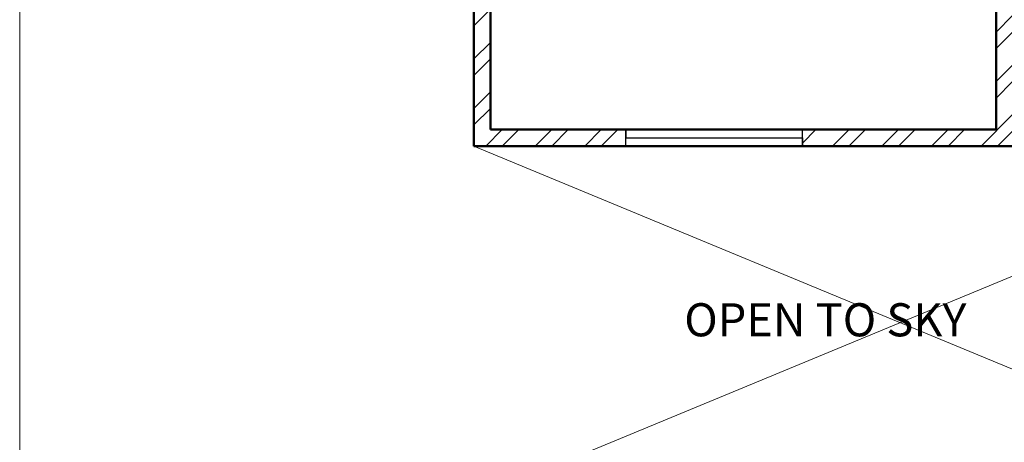
# Model space of a CAD drawing. Units: inches. Extents: x 1901 to 2863, y 888 to 2433.
# Tile 49 of 91: x 1901 to 2169, y 1732 to 1847. Entities that reach past the tile are written whole.
import ezdxf

# ---------------------------------------------------------------- set-up
doc = ezdxf.new("R2010")
doc.units = ezdxf.units.IN
for name, color, linetype, lineweight in [('A-ANNO-SYMB', 8, 'Continuous', 13), ('A-AREA-IDEN', 7, 'Continuous', 18), ('A-FLOR-FIXT', 9, 'Continuous', 18), ('A-GLAZ', 3, 'Continuous', 25), ('A-WALL', 7, 'Continuous', 50), ('A-WALL-PATT', 8, 'Continuous', 13)]:
    doc.layers.add(name, color=color, linetype=linetype, lineweight=lineweight)
doc.styles.get("Standard").update_dxf_attribs({"font": 'arial.ttf'})

# ---------------------------------------------------------------- blocks, each defined once
blk = doc.blocks.new('WIN-48')
for p, q in [((0, 2.25), (0, 4.5)), ((0, 4.5), (0, 0)), ((48, 4.5), (48, 0)), ((48, 2.25), (0, 2.25)), ((48, 0), (48, 2.25))]:
    blk.add_line(p, q)

msp = doc.modelspace()

# ---------------------------------------------------------------- hatches: boundary and pattern name
at = {"layer": 'A-WALL-PATT'}
h = msp.add_hatch(dxfattribs=at)
h.set_pattern_fill('ANSI32', color=256)
h.paths.add_polyline_path([(2192.5, 2274.13), (2141.26, 2274.13), (2141.26, 2269.63), (2192.5, 2269.63)])
h.paths.add_polyline_path([(2259.93, 2274.13), (2216.5, 2274.13), (2216.5, 2269.63), (2255.43, 2269.63), (2255.43, 2214.63), (2250.81, 2214.63), (2250.81, 2210.13), (2259.93, 2210.13), (2259.93, 2215.13), (2271.76, 2215.13), (2271.76, 2217.38), (2271.76, 2219.63), (2259.93, 2219.63)])
h.paths.add_polyline_path([(2171.43, 2269.63), (2166.93, 2269.63), (2166.93, 2219.63), (2121.24, 2219.63), (2121.24, 2215.13), (2166.93, 2215.13), (2166.93, 2083.13), (2161.81, 2083.13), (2161.81, 2078.63), (2171.43, 2078.63), (2177, 2078.63), (2177, 2080.88), (2177, 2083.13), (2171.43, 2083.13), (2171.43, 2210.13), (2230.91, 2210.13), (2230.91, 2212.38), (2230.91, 2214.63), (2171.43, 2214.63)])
h.paths.add_polyline_path([(2117.26, 2274.13), (2089.43, 2274.13), (2089.43, 2219.63), (2081.14, 2219.63), (2081.14, 2215.13), (2089.43, 2215.13), (2098, 2215.13), (2098, 2217.38), (2098, 2219.63), (2093.93, 2219.63), (2093.93, 2269.63), (2117.26, 2269.63), (2117.26, 2271.88)])
h.paths.add_polyline_path([(2343.43, 2219.63), (2329.29, 2219.63), (2329.29, 2215.13), (2338.93, 2215.13), (2338.93, 2184.74), (2343.43, 2184.74)])
h.paths.add_polyline_path([(2338.93, 2083.13), (2329.29, 2083.13), (2208.97, 2083.13), (2208.97, 2078.63), (2338.93, 2078.63)])
h.paths.add_polyline_path([(2343.43, 2136.74), (2338.93, 2136.74), (2338.93, 1872.63), (2343.43, 1872.63)])
h.paths.add_polyline_path([(2343.43, 1863.63), (2397.68, 1863.63), (2397.68, 1821.63), (2384.14, 1821.63), (2384.14, 1812.63), (2418.33, 1812.63), (2418.33, 1817.13), (2418.33, 1821.63), (2406.68, 1821.63), (2406.68, 1863.63), (2459.5, 1863.63), (2459.5, 1821.63), (2447.14, 1821.63), (2447.14, 1812.63), (2459.5, 1812.63), (2468.5, 1812.63), (2468.5, 1872.63), (2394.43, 1872.63), (2334.43, 1872.63), (2334.43, 1812.63), (2343.43, 1812.63), (2353.25, 1812.63), (2353.25, 1821.63), (2343.43, 1821.63)])
h.paths.add_polyline_path([(2510.01, 1872.63), (2468.5, 1872.63), (2468.5, 1868.13), (2510.01, 1868.13)])
h.paths.add_polyline_path([(2514.01, 1817.13), (2468.5, 1817.13), (2468.5, 1812.63), (2482.11, 1812.63), (2482.11, 1800.61), (2486.61, 1800.61), (2486.61, 1812.63), (2514.01, 1812.63)])
h.paths.add_polyline_path([(2299.25, 1814.88), (2299.25, 1817.13), (2295.93, 1817.13), (2295.93, 1854.17), (2293.68, 1854.17), (2291.43, 1854.17), (2291.43, 1817.13), (2266.11, 1817.13), (2266.11, 1812.63), (2299.25, 1812.63)])
h.paths.add_polyline_path([(2218.11, 1817.13), (2206.46, 1817.13), (2171.43, 1817.13), (2171.43, 1949.13), (2190.1, 1949.13), (2190.1, 1953.63), (2163.47, 1953.63), (2163.47, 1949.13), (2166.93, 1949.13), (2166.93, 1817.13), (2114.3, 1817.13), (2114.3, 1812.63), (2218.11, 1812.63)])
h.paths.add_polyline_path([(2029.43, 1970.92), (2024.93, 1970.92), (2024.93, 1912.72), (2029.43, 1912.72)])
h.paths.add_polyline_path([(2132.3, 1953.63), (2113.93, 1953.63), (2113.93, 1975.89), (2111.68, 1975.89), (2109.43, 1975.89), (2109.43, 1953.63), (2029.43, 1953.63), (2029.43, 1949.13), (2132.3, 1949.13)])
h.paths.add_polyline_path([(2029.43, 1853.61), (2029.31, 1853.61), (2029.31, 1853.61), (2029.43, 1853.61), (2029.43, 1864.72), (2024.93, 1864.72), (2024.93, 1812.63), (2066.3, 1812.63), (2066.3, 1814.88), (2066.3, 1817.13), (2029.43, 1817.13)])
h.paths.add_polyline_path([(2122.93, 2010.09), (2120.68, 2010.09), (2118.43, 2010.09), (2118.43, 2006.13), (2029.43, 2006.13), (2029.43, 2001.63), (2109.43, 2001.63), (2109.43, 1998.04), (2113.93, 1998.04), (2113.93, 2001.63), (2122.93, 2001.63)])
h.paths.add_polyline_path([(2029.43, 2031.38), (2024.93, 2031.38), (2024.93, 1994.92), (2027.18, 1994.92), (2029.43, 1994.92)])
h.paths.add_polyline_path([(2029.43, 2136.74), (2024.93, 2136.74), (2024.93, 2067.38), (2027.18, 2067.38), (2029.43, 2067.38)])
h.paths.add_polyline_path([(2125.62, 2083.13), (2029.43, 2083.13), (2029.43, 2078.63), (2118.43, 2078.63), (2118.43, 2030.71), (2122.93, 2030.71), (2122.93, 2078.63), (2125.62, 2078.63)])
h.paths.add_polyline_path([(2029.43, 2215.13), (2040.47, 2215.13), (2040.47, 2217.38), (2040.47, 2219.63), (2024.93, 2219.63), (2024.93, 2184.74), (2029.43, 2184.74), (2029.43, 2187.78)])
h.paths.add_polyline_path([(2686.43, 2274.13), (2659.28, 2274.13), (2659.28, 2269.63), (2681.93, 2269.63), (2681.93, 2219.63), (2676.82, 2219.63), (2676.82, 2215.13), (2681.93, 2215.13), (2697.01, 2215.13), (2697.01, 2217.38), (2697.01, 2219.63), (2686.43, 2219.63)])
h.paths.add_polyline_path([(2609.93, 2269.63), (2635.28, 2269.63), (2635.28, 2274.13), (2571.43, 2274.13), (2571.43, 2269.63), (2605.43, 2269.63), (2605.43, 2214.63), (2549.1, 2214.63), (2549.1, 2210.13), (2605.43, 2210.13), (2605.43, 2083.13), (2601.01, 2083.13), (2601.01, 2080.88), (2601.01, 2078.63), (2609.93, 2078.63), (2616.16, 2078.63), (2616.16, 2080.88), (2616.16, 2083.13), (2609.93, 2083.13), (2609.93, 2215.13), (2651.46, 2215.13), (2651.46, 2217.38), (2651.46, 2219.63), (2609.93, 2219.63)])
h.paths.add_polyline_path([(2521.43, 2269.63), (2547.43, 2269.63), (2547.43, 2271.88), (2547.43, 2274.13), (2516.93, 2274.13), (2516.93, 2219.63), (2506.41, 2219.63), (2506.41, 2215.13), (2516.93, 2215.13), (2516.93, 2210.13), (2525.4, 2210.13), (2525.4, 2212.38), (2525.4, 2214.63), (2521.43, 2214.63)])
h.paths.add_polyline_path([(2456.01, 2219.63), (2439.43, 2219.63), (2439.43, 2187.89), (2443.93, 2187.89), (2443.93, 2215.13), (2456.01, 2215.13)])
h.paths.add_polyline_path([(2752.93, 2219.63), (2739.48, 2219.63), (2739.48, 2215.13), (2748.43, 2215.13), (2748.43, 2187.89), (2752.93, 2187.89)])
h.paths.add_polyline_path([(2752.93, 2139.89), (2748.43, 2139.89), (2748.43, 2083.13), (2648.42, 2083.13), (2648.42, 2078.63), (2654.93, 2078.63), (2654.93, 2039.44), (2659.43, 2039.44), (2659.43, 2078.63), (2748.43, 2078.63), (2748.43, 2063.43), (2752.93, 2063.43)])
h.paths.add_polyline_path([(2752.93, 2010.63), (2659.43, 2010.63), (2659.43, 2015.65), (2654.93, 2015.65), (2654.93, 2010.63), (2605.43, 2010.63), (2605.43, 1920.97), (2609.93, 1920.97), (2609.93, 2006.13), (2748.43, 2006.13), (2748.43, 1982.47), (2752.93, 1982.47)])
h.paths.add_polyline_path([(2752.93, 2027.43), (2748.43, 2027.43), (2748.43, 2010.63), (2752.93, 2010.63)])
h.paths.add_polyline_path([(2748.43, 1886.13), (2609.93, 1886.13), (2609.93, 1889.72), (2605.43, 1889.72), (2605.43, 1861.26), (2609.93, 1861.26), (2609.93, 1881.63), (2748.43, 1881.63)])
h.paths.add_polyline_path([(2456.86, 2228.83), (2498.4, 2228.83), (2498.4, 2247.49), (2456.86, 2247.49)], flags=9)
h.paths.add_polyline_path([(2038.6, 2237.42), (2080.17, 2237.42), (2080.17, 2256.08), (2038.6, 2256.08)], flags=9)
h.paths.add_polyline_path([(2292.01, 1062.39), (2539.93, 1062.39), (2539.93, 1099.49), (2292.01, 1099.49)], flags=9)
h.paths.add_polyline_path([(2424.91, 1832.25), (2448.51, 1832.25), (2448.51, 1846.68), (2424.91, 1846.68)], flags=25)
h.paths.add_polyline_path([(2359.08, 1832.25), (2382.68, 1832.25), (2382.68, 1846.68), (2359.08, 1846.68)], flags=25)
h.paths.add_polyline_path([(2352.9, 1684.8), (2367.54, 1684.8), (2367.54, 1697.17), (2352.9, 1697.17)], flags=9)
h.paths.add_polyline_path([(2079.29, 1755.83), (2169.02, 1755.83), (2169.02, 1774.37), (2079.29, 1774.37)], flags=9)
h.paths.add_polyline_path([(2404.09, 1373.86), (2404.09, 1463.59), (2385.54, 1463.59), (2385.54, 1373.86)], flags=9)
h.paths.add_polyline_path([(2268.09, 2236.37), (2309.64, 2236.37), (2309.64, 2255.03), (2268.09, 2255.03)], flags=9)
h.paths.add_polyline_path([(2575.96, 1700.95), (2665.7, 1700.95), (2665.7, 1719.5), (2575.96, 1719.5)], flags=9)
h.paths.add_polyline_path([(2302.96, 1878.47), (2329.52, 1878.47), (2329.52, 1888.78), (2302.96, 1888.78)], flags=9)
h.paths.add_polyline_path([(2097.42, 2240.58), (2126.57, 2240.58), (2126.57, 2259.23), (2097.42, 2259.23)], flags=9)
h.paths.add_polyline_path([(2208.72, 2246.12), (2237.88, 2246.12), (2237.88, 2264.78), (2208.72, 2264.78)], flags=9)
h.paths.add_polyline_path([(2038.15, 1925.96), (2076.99, 1925.96), (2076.99, 1944.62), (2038.15, 1944.62)], flags=9)
h.paths.add_polyline_path([(2239.14, 1926.67), (2288.46, 1926.67), (2288.46, 1945.33), (2239.14, 1945.33)], flags=9)
h.paths.add_polyline_path([(2175.43, 2007.33), (2212.36, 2007.33), (2212.36, 2025.99), (2175.43, 2025.99)], flags=9)
h.paths.add_polyline_path([(2225.03, 2091.79), (2263.87, 2091.79), (2263.87, 2110.45), (2225.03, 2110.45)], flags=9)
h.paths.add_polyline_path([(2035.4, 2098.48), (2074.24, 2098.48), (2074.24, 2117.14), (2035.4, 2117.14)], flags=9)
h.paths.add_polyline_path([(2050.1, 2029.21), (2083.26, 2029.21), (2083.26, 2047.87), (2050.1, 2047.87)], flags=9)
h.paths.add_polyline_path([(2069.68, 1956.72), (2098.83, 1956.72), (2098.83, 1975.38), (2069.68, 1975.38)], flags=25)
h.paths.add_polyline_path([(2328.62, 1753.34), (2361.66, 1753.34), (2361.66, 1771.99), (2328.62, 1771.99)], flags=9)
h.paths.add_polyline_path([(2395.16, 2060.89), (2395.16, 2140.65), (2378.68, 2140.65), (2378.68, 2060.89)], flags=9)
h.paths.add_polyline_path([(2463.73, 2059.02), (2492.89, 2059.02), (2492.89, 2077.68), (2463.73, 2077.68)], flags=9)
h.paths.add_polyline_path([(2458.03, 2181.54), (2496.87, 2181.54), (2496.87, 2200.19), (2458.03, 2200.19)], flags=9)
h.paths.add_polyline_path([(2527.58, 2243.07), (2556.73, 2243.07), (2556.73, 2261.73), (2527.58, 2261.73)], flags=9)
h.paths.add_polyline_path([(2694.46, 2232.77), (2736.03, 2232.77), (2736.03, 2251.42), (2694.46, 2251.42)], flags=9)
h.paths.add_polyline_path([(2637.82, 2249.22), (2666.98, 2249.22), (2666.98, 2267.88), (2637.82, 2267.88)], flags=9)
h.paths.add_polyline_path([(2623.69, 2183.54), (2662.53, 2183.54), (2662.53, 2202.2), (2623.69, 2202.2)], flags=9)
h.paths.add_polyline_path([(2691.97, 2021.5), (2725.12, 2021.5), (2725.12, 2040.16), (2691.97, 2040.16)], flags=9)
h.paths.add_polyline_path([(2621.04, 1975.91), (2662.34, 1975.91), (2662.34, 1994.57), (2621.04, 1994.57)], flags=25)
h.paths.add_polyline_path([(2479.03, 1927.62), (2519.84, 1927.62), (2519.84, 1946.28), (2479.03, 1946.28)], flags=9)
h.paths.add_polyline_path([(2670.94, 1849.08), (2716.01, 1849.08), (2716.01, 1867.73), (2670.94, 1867.73)], flags=9)
h.paths.add_polyline_path([(2523.61, 1782.96), (2550.17, 1782.96), (2550.17, 1793.26), (2523.61, 1793.26)], flags=9)
h.paths.add_polyline_path([(2450.84, 1207.33), (2492.39, 1207.33), (2492.39, 1225.99), (2450.84, 1225.99)], flags=9)
h.paths.add_polyline_path([(2527.75, 1203.84), (2556.91, 1203.84), (2556.91, 1222.5), (2527.75, 1222.5)], flags=9)
h.paths.add_polyline_path([(2639.11, 1207.2), (2668.27, 1207.2), (2668.27, 1225.86), (2639.11, 1225.86)], flags=9)
h.paths.add_polyline_path([(2692.59, 1218.97), (2734.17, 1218.97), (2734.17, 1237.62), (2692.59, 1237.62)], flags=9)
h.paths.add_polyline_path([(2669.27, 1366.33), (2708.11, 1366.33), (2708.11, 1384.99), (2669.27, 1384.99)], flags=9)
h.paths.add_polyline_path([(2463.31, 1358.03), (2502.15, 1358.03), (2502.15, 1376.69), (2463.31, 1376.69)], flags=9)
h.paths.add_polyline_path([(2494.72, 1449.96), (2531.65, 1449.96), (2531.65, 1468.62), (2494.72, 1468.62)], flags=9)
h.paths.add_polyline_path([(2675.57, 1422.16), (2708.72, 1422.16), (2708.72, 1440.81), (2675.57, 1440.81)], flags=9)
h.paths.add_polyline_path([(2685.63, 1493.89), (2714.79, 1493.89), (2714.79, 1512.55), (2685.63, 1512.55)], flags=9)
h.paths.add_polyline_path([(2686.8, 1529.91), (2725.65, 1529.91), (2725.65, 1548.57), (2686.8, 1548.57)], flags=9)
h.paths.add_polyline_path([(2503.65, 1537.99), (2552.97, 1537.99), (2552.97, 1556.65), (2503.65, 1556.65)], flags=9)
h.paths.add_polyline_path([(2291.71, 1643.5), (2318.28, 1643.5), (2318.28, 1653.81), (2291.71, 1653.81)], flags=9)
h.paths.add_polyline_path([(2450.63, 1610.52), (2477.19, 1610.52), (2477.19, 1620.82), (2450.63, 1620.82)], flags=9)
h.paths.add_polyline_path([(2359.99, 1551.81), (2422.25, 1551.81), (2422.25, 1562.12), (2359.99, 1562.12)], flags=9)
h.paths.add_polyline_path([(2280.11, 1249.01), (2321.65, 1249.01), (2321.65, 1267.66), (2280.11, 1267.66)], flags=9)
h.paths.add_polyline_path([(2164.06, 1274.23), (2193.22, 1274.23), (2193.22, 1292.89), (2164.06, 1292.89)], flags=9)
h.paths.add_polyline_path([(2118.21, 1277.69), (2151.25, 1277.69), (2151.25, 1296.35), (2118.21, 1296.35)], flags=9)
h.paths.add_polyline_path([(2031.95, 1268.53), (2073.52, 1268.53), (2073.52, 1287.19), (2031.95, 1287.19)], flags=9)
h.paths.add_polyline_path([(2050.2, 1409.08), (2089.04, 1409.08), (2089.04, 1427.74), (2050.2, 1427.74)], flags=9)
h.paths.add_polyline_path([(2243.74, 1421.03), (2282.58, 1421.03), (2282.58, 1439.69), (2243.74, 1439.69)], flags=9)
h.paths.add_polyline_path([(2190.75, 1509.77), (2231.56, 1509.77), (2231.56, 1528.43), (2190.75, 1528.43)], flags=9)
h.paths.add_polyline_path([(2058.39, 1475.42), (2091.55, 1475.42), (2091.55, 1494.07), (2058.39, 1494.07)], flags=9)
h.paths.add_polyline_path([(2062.45, 1553.09), (2091.6, 1553.09), (2091.6, 1571.75), (2062.45, 1571.75)], flags=9)
h.paths.add_polyline_path([(2219.52, 1590.37), (2266.15, 1590.37), (2266.15, 1609.02), (2219.52, 1609.02)], flags=9)
h.paths.add_polyline_path([(2041.07, 1584.19), (2079.91, 1584.19), (2079.91, 1602.85), (2041.07, 1602.85)], flags=9)
h = msp.add_hatch(dxfattribs=at)
h.set_pattern_fill('ANSI32', color=256)
h.paths.add_polyline_path([(2443.93, 2139.89), (2439.43, 2139.89), (2439.43, 2069.35), (2441.68, 2069.35), (2443.93, 2069.35), (2443.93, 2078.63), (2521.93, 2078.63), (2521.93, 2075.07), (2524.18, 2075.07), (2526.43, 2075.07), (2526.43, 2078.63), (2571.75, 2078.63), (2571.75, 2080.88), (2571.75, 2083.13), (2443.93, 2083.13)])
h.paths.add_polyline_path([(2526.43, 2054.63), (2524.18, 2054.63), (2521.93, 2054.63), (2521.93, 2030.63), (2443.93, 2030.63), (2443.93, 2045.35), (2439.43, 2045.35), (2439.43, 1983.87), (2443.93, 1983.87), (2443.93, 2026.13), (2521.93, 2026.13), (2526.43, 2026.13)])
h.paths.add_polyline_path([(2443.93, 1923.87), (2439.43, 1923.87), (2439.43, 1872.63), (2443.93, 1872.63)])
h.paths.add_polyline_path([(2636.23, 1766.13), (2609.93, 1766.13), (2609.93, 1779.79), (2605.43, 1779.79), (2605.43, 1766.13), (2486.61, 1766.13), (2486.61, 1770.67), (2482.11, 1770.67), (2482.11, 1766.13), (2482.11, 1761.63), (2636.23, 1761.63), (2636.23, 1763.88)])
h.paths.add_polyline_path([(2519.54, 1663.38), (2519.54, 1665.63), (2494.93, 1665.63), (2481.83, 1665.63), (2481.83, 1663.38), (2481.83, 1661.13), (2490.43, 1661.13), (2490.43, 1640.16), (2494.93, 1640.16), (2494.93, 1661.13), (2519.54, 1661.13)])
h.paths.add_polyline_path([(2443.93, 1712.13), (2443.93, 1716.63), (2414.46, 1716.63), (2414.46, 1712.13), (2439.43, 1712.13), (2439.43, 1545.51), (2443.93, 1545.51), (2443.93, 1661.13), (2448.47, 1661.13), (2448.47, 1665.63), (2443.93, 1665.63)])
h.paths.add_polyline_path([(2343.43, 1712.13), (2365.52, 1712.13), (2365.52, 1714.38), (2365.52, 1716.63), (2333.87, 1716.63), (2333.87, 1714.38), (2333.87, 1712.13), (2338.93, 1712.13), (2338.93, 1575.63), (2338.93, 1545.51), (2343.43, 1545.51), (2343.43, 1547.51), (2343.43, 1580.13)])
h.paths.add_polyline_path([(2752.93, 1665.63), (2579.54, 1665.63), (2579.54, 1661.13), (2615.93, 1661.13), (2615.93, 1529.13), (2598.93, 1529.13), (2598.93, 1524.63), (2623.13, 1524.63), (2623.13, 1526.88), (2623.13, 1529.13), (2620.43, 1529.13), (2620.43, 1661.13), (2748.43, 1661.13), (2748.43, 1633.5), (2752.93, 1633.5)])
h.paths.add_polyline_path([(2752.93, 1419.93), (2748.43, 1419.93), (2748.43, 1400.13), (2659.43, 1400.13), (2659.43, 1444.33), (2657.18, 1444.33), (2654.93, 1444.33), (2654.93, 1400.13), (2643.65, 1400.13), (2643.65, 1395.63), (2748.43, 1395.63), (2748.43, 1364.04), (2752.93, 1364.04)])
h.paths.add_polyline_path([(2752.93, 1492.88), (2748.43, 1492.88), (2748.43, 1476.63), (2667.43, 1476.63), (2667.43, 1479.71), (2665.18, 1479.71), (2662.93, 1479.71), (2662.93, 1476.63), (2654.93, 1476.63), (2654.93, 1469.54), (2659.43, 1469.54), (2659.43, 1472.13), (2748.43, 1472.13), (2748.43, 1455.93), (2752.93, 1455.93)])
h.paths.add_polyline_path([(2752.93, 1304.04), (2748.43, 1304.04), (2748.43, 1263.63), (2738.66, 1263.63), (2738.66, 1259.13), (2752.93, 1259.13)])
h.paths.add_polyline_path([(2685.93, 1259.13), (2695.49, 1259.13), (2695.49, 1261.38), (2695.49, 1263.63), (2677.84, 1263.63), (2677.84, 1261.38), (2677.84, 1259.13), (2681.43, 1259.13), (2681.43, 1203.63), (2653.28, 1203.63), (2653.28, 1199.13), (2685.93, 1199.13), (2685.93, 1203.63)])
h.paths.add_polyline_path([(2609.43, 1395.63), (2611.85, 1395.63), (2611.85, 1400.13), (2598.89, 1400.13), (2598.89, 1397.88), (2598.89, 1395.63), (2604.93, 1395.63), (2604.93, 1268.13), (2554.73, 1268.13), (2554.73, 1265.88), (2554.73, 1263.63), (2604.93, 1263.63), (2604.93, 1203.63), (2571.31, 1203.63), (2571.31, 1199.13), (2604.93, 1199.13), (2629.28, 1199.13), (2629.28, 1201.38), (2629.28, 1203.63), (2609.43, 1203.63), (2609.43, 1258.63), (2609.43, 1259.13), (2654.8, 1259.13), (2654.8, 1263.63), (2609.43, 1263.63)])
h.paths.add_polyline_path([(2443.93, 1304.04), (2439.43, 1304.04), (2439.43, 1259.13), (2443.93, 1259.13), (2456.16, 1259.13), (2456.16, 1261.38), (2456.16, 1263.63), (2443.93, 1263.63)])
h.paths.add_polyline_path([(2525.43, 1263.63), (2531.78, 1263.63), (2531.78, 1268.13), (2520.93, 1268.13), (2520.93, 1263.63), (2511.41, 1263.63), (2511.41, 1259.13), (2520.93, 1259.13), (2520.93, 1199.13), (2547.31, 1199.13), (2547.31, 1201.38), (2547.31, 1203.63), (2525.43, 1203.63)])
h.paths.add_polyline_path([(2443.93, 1434.84), (2439.43, 1434.84), (2439.43, 1364.04), (2441.68, 1364.04), (2443.93, 1364.04)])
h.paths.add_polyline_path([(2567.13, 1400.13), (2443.93, 1400.13), (2443.93, 1395.63), (2567.13, 1395.63)])
h.paths.add_polyline_path([(2443.93, 1545.51), (2439.43, 1545.51), (2439.43, 1494.84), (2443.93, 1494.84)])
h.paths.add_polyline_path([(2494.93, 1553.35), (2492.68, 1553.35), (2490.43, 1553.35), (2490.43, 1524.63), (2494.93, 1524.63), (2525.94, 1524.63), (2525.94, 1526.88), (2525.94, 1529.13), (2494.93, 1529.13)])
h.paths.add_polyline_path([(2752.93, 1573.5), (2748.43, 1573.5), (2748.43, 1529.13), (2657.76, 1529.13), (2657.76, 1524.63), (2662.93, 1524.63), (2662.93, 1498.63), (2667.43, 1498.63), (2667.43, 1524.63), (2748.43, 1524.63), (2748.43, 1516.88), (2752.93, 1516.88)])
h.paths.add_polyline_path([(2038.6, 2237.42), (2080.17, 2237.42), (2080.17, 2256.08), (2038.6, 2256.08)], flags=9)
h.paths.add_polyline_path([(2292.01, 1062.39), (2539.93, 1062.39), (2539.93, 1099.49), (2292.01, 1099.49)], flags=9)
h.paths.add_polyline_path([(2424.91, 1832.25), (2448.51, 1832.25), (2448.51, 1846.68), (2424.91, 1846.68)], flags=9)
h.paths.add_polyline_path([(2359.08, 1832.25), (2382.68, 1832.25), (2382.68, 1846.68), (2359.08, 1846.68)], flags=9)
h.paths.add_polyline_path([(2352.9, 1684.8), (2367.54, 1684.8), (2367.54, 1697.17), (2352.9, 1697.17)], flags=9)
h.paths.add_polyline_path([(2079.29, 1755.83), (2169.02, 1755.83), (2169.02, 1774.37), (2079.29, 1774.37)], flags=9)
h.paths.add_polyline_path([(2404.09, 1373.86), (2404.09, 1463.59), (2385.54, 1463.59), (2385.54, 1373.86)], flags=9)
h.paths.add_polyline_path([(2268.09, 2236.37), (2309.64, 2236.37), (2309.64, 2255.03), (2268.09, 2255.03)], flags=9)
h.paths.add_polyline_path([(2575.96, 1700.95), (2665.7, 1700.95), (2665.7, 1719.5), (2575.96, 1719.5)], flags=9)
h.paths.add_polyline_path([(2302.96, 1878.47), (2329.52, 1878.47), (2329.52, 1888.78), (2302.96, 1888.78)], flags=9)
h.paths.add_polyline_path([(2097.42, 2240.58), (2126.57, 2240.58), (2126.57, 2259.23), (2097.42, 2259.23)], flags=9)
h.paths.add_polyline_path([(2208.72, 2246.12), (2237.88, 2246.12), (2237.88, 2264.78), (2208.72, 2264.78)], flags=9)
h.paths.add_polyline_path([(2038.15, 1925.96), (2076.99, 1925.96), (2076.99, 1944.62), (2038.15, 1944.62)], flags=9)
h.paths.add_polyline_path([(2239.14, 1926.67), (2288.46, 1926.67), (2288.46, 1945.33), (2239.14, 1945.33)], flags=9)
h.paths.add_polyline_path([(2175.43, 2007.33), (2212.36, 2007.33), (2212.36, 2025.99), (2175.43, 2025.99)], flags=9)
h.paths.add_polyline_path([(2225.03, 2091.79), (2263.87, 2091.79), (2263.87, 2110.45), (2225.03, 2110.45)], flags=9)
h.paths.add_polyline_path([(2035.4, 2098.48), (2074.24, 2098.48), (2074.24, 2117.14), (2035.4, 2117.14)], flags=9)
h.paths.add_polyline_path([(2050.1, 2029.21), (2083.26, 2029.21), (2083.26, 2047.87), (2050.1, 2047.87)], flags=9)
h.paths.add_polyline_path([(2069.68, 1956.72), (2098.83, 1956.72), (2098.83, 1975.38), (2069.68, 1975.38)], flags=9)
h.paths.add_polyline_path([(2328.62, 1753.34), (2361.66, 1753.34), (2361.66, 1771.99), (2328.62, 1771.99)], flags=9)
h.paths.add_polyline_path([(2395.16, 2060.89), (2395.16, 2140.65), (2378.68, 2140.65), (2378.68, 2060.89)], flags=9)
h.paths.add_polyline_path([(2463.73, 2059.02), (2492.89, 2059.02), (2492.89, 2077.68), (2463.73, 2077.68)], flags=9)
h.paths.add_polyline_path([(2458.03, 2181.54), (2496.87, 2181.54), (2496.87, 2200.19), (2458.03, 2200.19)], flags=9)
h.paths.add_polyline_path([(2456.86, 2228.83), (2498.4, 2228.83), (2498.4, 2247.49), (2456.86, 2247.49)], flags=9)
h.paths.add_polyline_path([(2527.58, 2243.07), (2556.73, 2243.07), (2556.73, 2261.73), (2527.58, 2261.73)], flags=9)
h.paths.add_polyline_path([(2694.46, 2232.77), (2736.03, 2232.77), (2736.03, 2251.42), (2694.46, 2251.42)], flags=9)
h.paths.add_polyline_path([(2637.82, 2249.22), (2666.98, 2249.22), (2666.98, 2267.88), (2637.82, 2267.88)], flags=9)
h.paths.add_polyline_path([(2623.69, 2183.54), (2662.53, 2183.54), (2662.53, 2202.2), (2623.69, 2202.2)], flags=9)
h.paths.add_polyline_path([(2691.97, 2021.5), (2725.12, 2021.5), (2725.12, 2040.16), (2691.97, 2040.16)], flags=9)
h.paths.add_polyline_path([(2621.04, 1975.91), (2662.34, 1975.91), (2662.34, 1994.57), (2621.04, 1994.57)], flags=9)
h.paths.add_polyline_path([(2479.03, 1927.62), (2519.84, 1927.62), (2519.84, 1946.28), (2479.03, 1946.28)], flags=9)
h.paths.add_polyline_path([(2670.94, 1849.08), (2716.01, 1849.08), (2716.01, 1867.73), (2670.94, 1867.73)], flags=9)
h.paths.add_polyline_path([(2523.61, 1782.96), (2550.17, 1782.96), (2550.17, 1793.26), (2523.61, 1793.26)], flags=9)
h.paths.add_polyline_path([(2450.84, 1207.33), (2492.39, 1207.33), (2492.39, 1225.99), (2450.84, 1225.99)], flags=9)
h.paths.add_polyline_path([(2527.75, 1203.84), (2556.91, 1203.84), (2556.91, 1222.5), (2527.75, 1222.5)], flags=9)
h.paths.add_polyline_path([(2639.11, 1207.2), (2668.27, 1207.2), (2668.27, 1225.86), (2639.11, 1225.86)], flags=9)
h.paths.add_polyline_path([(2692.59, 1218.97), (2734.17, 1218.97), (2734.17, 1237.62), (2692.59, 1237.62)], flags=9)
h.paths.add_polyline_path([(2669.27, 1366.33), (2708.11, 1366.33), (2708.11, 1384.99), (2669.27, 1384.99)], flags=25)
h.paths.add_polyline_path([(2463.31, 1358.03), (2502.15, 1358.03), (2502.15, 1376.69), (2463.31, 1376.69)], flags=9)
h.paths.add_polyline_path([(2494.72, 1449.96), (2531.65, 1449.96), (2531.65, 1468.62), (2494.72, 1468.62)], flags=9)
h.paths.add_polyline_path([(2675.57, 1422.16), (2708.72, 1422.16), (2708.72, 1440.81), (2675.57, 1440.81)], flags=25)
h.paths.add_polyline_path([(2685.63, 1493.89), (2714.79, 1493.89), (2714.79, 1512.55), (2685.63, 1512.55)], flags=9)
h.paths.add_polyline_path([(2686.8, 1529.91), (2725.65, 1529.91), (2725.65, 1548.57), (2686.8, 1548.57)], flags=25)
h.paths.add_polyline_path([(2503.65, 1537.99), (2552.97, 1537.99), (2552.97, 1556.65), (2503.65, 1556.65)], flags=9)
h.paths.add_polyline_path([(2291.71, 1643.5), (2318.28, 1643.5), (2318.28, 1653.81), (2291.71, 1653.81)], flags=9)
h.paths.add_polyline_path([(2450.63, 1610.52), (2477.19, 1610.52), (2477.19, 1620.82), (2450.63, 1620.82)], flags=9)
h.paths.add_polyline_path([(2359.99, 1551.81), (2422.25, 1551.81), (2422.25, 1562.12), (2359.99, 1562.12)], flags=9)
h.paths.add_polyline_path([(2280.11, 1249.01), (2321.65, 1249.01), (2321.65, 1267.66), (2280.11, 1267.66)], flags=9)
h.paths.add_polyline_path([(2164.06, 1274.23), (2193.22, 1274.23), (2193.22, 1292.89), (2164.06, 1292.89)], flags=9)
h.paths.add_polyline_path([(2118.21, 1277.69), (2151.25, 1277.69), (2151.25, 1296.35), (2118.21, 1296.35)], flags=9)
h.paths.add_polyline_path([(2031.95, 1268.53), (2073.52, 1268.53), (2073.52, 1287.19), (2031.95, 1287.19)], flags=9)
h.paths.add_polyline_path([(2050.2, 1409.08), (2089.04, 1409.08), (2089.04, 1427.74), (2050.2, 1427.74)], flags=9)
h.paths.add_polyline_path([(2243.74, 1421.03), (2282.58, 1421.03), (2282.58, 1439.69), (2243.74, 1439.69)], flags=9)
h.paths.add_polyline_path([(2190.75, 1509.77), (2231.56, 1509.77), (2231.56, 1528.43), (2190.75, 1528.43)], flags=9)
h.paths.add_polyline_path([(2058.39, 1475.42), (2091.55, 1475.42), (2091.55, 1494.07), (2058.39, 1494.07)], flags=9)
h.paths.add_polyline_path([(2062.45, 1553.09), (2091.6, 1553.09), (2091.6, 1571.75), (2062.45, 1571.75)], flags=9)
h.paths.add_polyline_path([(2219.52, 1590.37), (2266.15, 1590.37), (2266.15, 1609.02), (2219.52, 1609.02)], flags=9)
h.paths.add_polyline_path([(2041.07, 1584.19), (2079.91, 1584.19), (2079.91, 1602.85), (2041.07, 1602.85)], flags=9)

# ---------------------------------------------------------------- linework, layer by layer
at = {"layer": 'A-ANNO-SYMB'}
for p, q in [((2256.71, 1812.63), (2024.93, 1716.63)), ((2024.93, 1812.63), (2256.71, 1716.63))]:
    msp.add_line(p, q, dxfattribs=at)
at = {"layer": 'A-FLOR-FIXT'}
msp.add_lwpolyline([(1901.45, 2433.12), (2863.43, 2433.12), (2863.43, 961.82), (1901.45, 961.82)], close=True, dxfattribs=at)
at = {"layer": 'A-WALL'}
for p, q in [((2024.93, 2219.63), (2024.93, 1812.63)), ((2029.43, 2215.13), (2029.43, 1817.13)), ((2166.93, 1949.13), (2166.93, 1817.13)), ((2029.43, 1817.13), (2166.93, 1817.13)), ((2024.93, 1812.63), (2299.25, 1812.63))]:
    msp.add_line(p, q, dxfattribs=at)

# ---------------------------------------------------------------- block references
at = {"layer": 'A-GLAZ', "rotation": 180}
msp.add_blockref('WIN-48', (2114.3, 1817.13), dxfattribs=at)

# ---------------------------------------------------------------- texts
at = {"layer": 'A-AREA-IDEN', "insert": (2082.15, 1769.9), "char_height": 9, "attachment_point": 1}
msp.add_mtext_dynamic_manual_height_columns('OPEN TO SKY', width=233.3304, gutter_width=12.5, heights=[0], dxfattribs=at)

doc.saveas('drawing.dxf')
